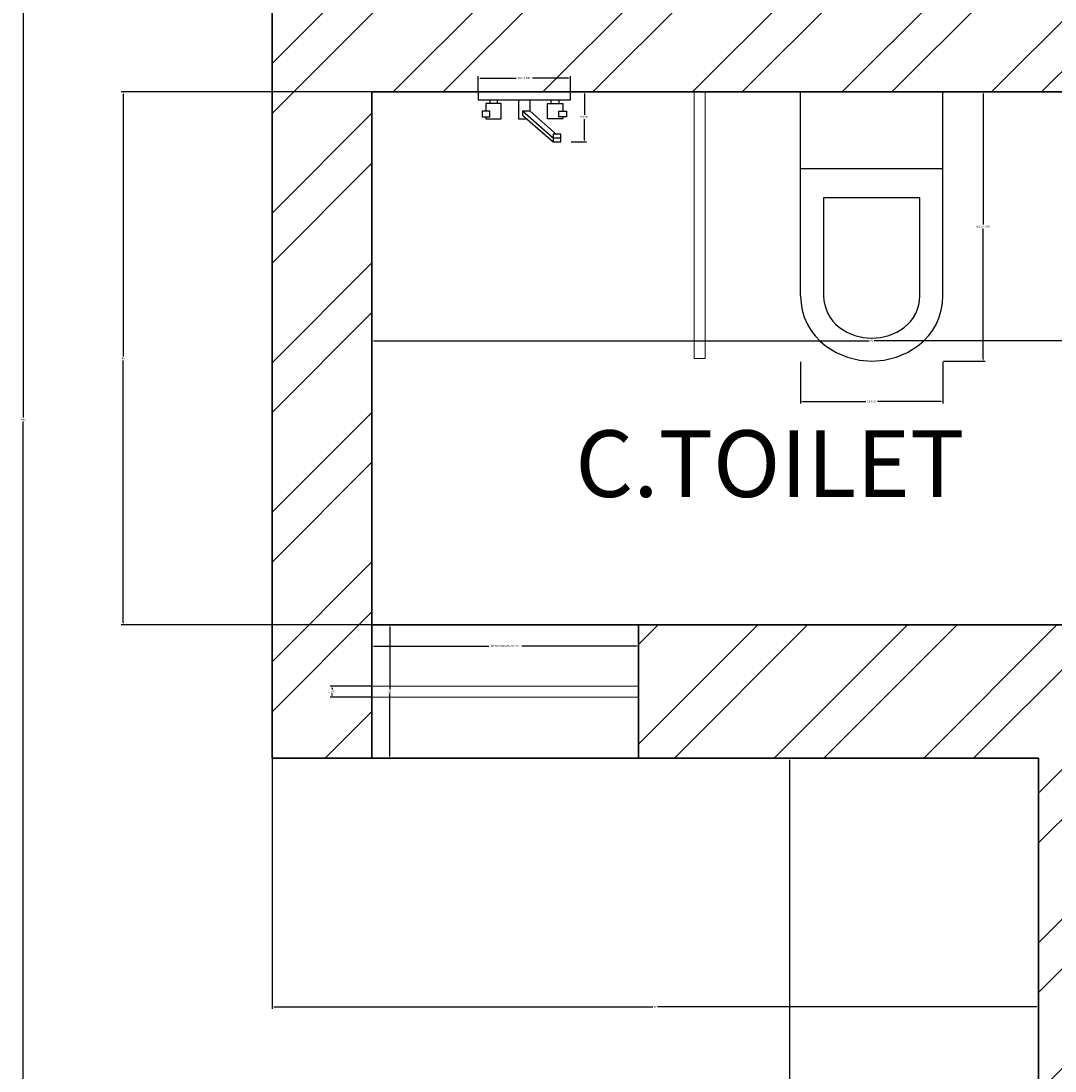
# Model space of a CAD drawing. Units: inches. Extents: x 3449 to 3843, y 1566 to 2054.
# Tile 2 of 8: x 3449 to 3543, y 1751 to 1846. Entities that reach past the tile are written whole.
import ezdxf

# ---------------------------------------------------------------- set-up
doc = ezdxf.new("R2010")
doc.units = ezdxf.units.IN
for name, color, linetype, lineweight in [('A-ANNO-DIMS', 2, 'Continuous', 18), ('A-AREA-IDEN', 7, 'Continuous', 25), ('A-GLAZ', 5, 'Continuous', 18), ('A-WALL', 7, 'Continuous', 35), ('A-WALL-PATT', 251, 'Continuous', 13), ('Сантехника', 7, 'Continuous', 18)]:
    doc.layers.add(name, color=color, linetype=linetype, lineweight=lineweight)
doc.layers.add('SANTEH', color=7, linetype='Continuous')
doc.styles.get("Standard").update_dxf_attribs({"font": 'arial.ttf'})
doc.dimstyles.get("Standard").update_dxf_attribs({"dimtxt": 0.18, "dimasz": 0.18, "dimexe": 0.18, "dimexo": 0.0625, "dimgap": 0.09, "dimtad": 0, "dimtih": 1, "dimtoh": 1, "dimdec": 4, "dimzin": 0, "dimdsep": 46, "dimtxsty": 'Standard', "dimcen": 0.09, "dimadec": 0, "dimazin": 0, "dimtfac": 1, "dimtdec": 4, "dimtofl": 0, "dimtmove": 0, "dimatfit": 3, "dimfxl": 1, "dimtolj": 1, "dimtzin": 0, "dimarcsym": 0})

# ---------------------------------------------------------------- blocks, each defined once
blk = doc.blocks.new('WC With Cistern_103')
at = {"layer": 'SANTEH'}
for p, q in [((0, 170), (0, 700)), ((370, 700), (0, 700)), ((370, 170), (370, 700)), ((370, 500), (0, 500)), ((60, 425), (60, 170)), ((310, 425), (60, 425)), ((310, 170), (310, 425))]:
    blk.add_line(p, q, dxfattribs=at)
for points in [[(0, 170), (1.1, 151.2), (4.3, 132.7), (9.7, 114.6), (17.1, 97.3), (26.5, 81), (37.7, 65.9), (50.6, 52.1), (65, 40)], [(60, 170), (60.7, 158.1), (62.7, 146.5), (66.1, 135.1), (70.8, 124.2), (76.7, 113.9), (83.8, 104.3), (91.9, 95.7), (101, 88)], [(269, 88), (278.1, 95.7), (286.2, 104.3), (293.3, 113.9), (299.2, 124.2), (303.9, 135.1), (307.3, 146.5), (309.3, 158.1), (310, 170)], [(305, 40), (319.4, 52.1), (332.3, 65.9), (343.5, 81), (352.9, 97.3), (360.3, 114.6), (365.7, 132.7), (368.9, 151.2), (370, 170)], [(101, 88), (120, 76), (140.7, 67.2), (162.6, 61.8), (185, 60), (207.4, 61.8), (229.3, 67.2), (250, 76), (269, 88)], [(65, 40), (92.2, 22.8), (121.8, 10.3), (153, 2.6), (185, 0), (217, 2.6), (248.2, 10.3), (277.8, 22.8), (305, 40)]]:
    blk.add_lwpolyline(points, dxfattribs=at)
blk = doc.blocks.new('Faucet - kit sink front')
at = {"layer": 'SANTEH'}
for p, q in [((-0.25, 3), (3.75, 6.5)), ((3.75, 6), (-0.25, 2.5)), ((4.1921, 5.5041), (0.75, 2.5)), ((3.75, 6), (3.75, 6.5)), ((3.75, 6.5), (4.75, 6.5)), ((3.75, 5.5), (3.75, 6)), ((4.75, 6), (3.75, 6)), ((4.75, 5.5), (3.75, 5.5)), ((4.75, 6.5), (4.75, 6)), ((4.75, 6), (4.75, 5.5)), ((-0.75, 3.5), (0.3192, 3.5)), ((-0.75, 1), (-0.75, 3.5)), ((-0.25, 2.5), (-0.25, 3)), ((-4.5, 1), (-4.5, 1.5)), ((-3.5, 1.5), (-3.5, 1)), ((0.75, 2.5), (-0.25, 2.5)), ((0.75, 2.5), (0.75, 1)), ((3.5, 1.5), (3.5, 1)), ((4.5, 1), (4.5, 1.5))]:
    blk.add_line(p, q, dxfattribs=at)
for points in [[(-5.5, 2.5), (-5.5, 3.25), (-4.5, 3.25), (-4.5, 2.5)], [(5.5, 2.5), (5.5, 3.25), (4.5, 3.25), (4.5, 2.5)], [(-6, 0), (-6, 1), (6, 1), (6, 0)]]:
    blk.add_lwpolyline(points, close=True, dxfattribs=at)
for points in [[(-5, 3.2513), (-5, 3.5), (-3, 3.5), (-3, 1.5), (-5, 1.5), (-5, 2.5)], [(5, 3.2513), (5, 3.5), (3, 3.5), (3, 1.5), (5, 1.5), (5, 2.5)]]:
    blk.add_lwpolyline(points, dxfattribs=at)
blk = doc.blocks.new('SHOWER-SCREEN-24')
for p, q in [((0, 24), (0, 0)), ((1, 24), (1, 0)), ((0, 0), (1, 0))]:
    blk.add_line(p, q)
blk = doc.blocks.new('GLAZING-24')
for p, q in [((24, 1), (0, 1)), ((24, 0), (0, 0))]:
    blk.add_line(p, q)
blk = doc.blocks.new('*D50')
at = {"layer": 'A-ANNO-DIMS', "color": 0, "lineweight": -2, "transparency": 16777216}
for p, q in [((3532.56, 1839.614), (3536.315, 1839.614)), ((3536.135, 1839.434), (3536.135, 1827.673)), ((3536.135, 1815.545), (3536.135, 1827.307)), ((3532.56, 1815.365), (3536.315, 1815.365))]:
    blk.add_line(p, q, dxfattribs=at)
at = {"layer": 'A-ANNO-DIMS', "color": 0, "transparency": 16777216}
for points in [[(3536.105, 1839.434), (3536.165, 1839.434), (3536.135, 1839.614)], [(3536.105, 1815.545), (3536.165, 1815.545), (3536.135, 1815.365)]]:
    blk.add_solid(points, dxfattribs=at)
at = {"layer": 'Defpoints', "color": 0, "transparency": 16777216}
for p in [(3532.497, 1839.614), (3536.135, 1839.614), (3532.497, 1815.365)]:
    blk.add_point(p, dxfattribs=at)
at = {"layer": 'A-ANNO-DIMS', "color": 0, "transparency": 16777216, "insert": (3536.135, 1827.49), "char_height": 0.18, "attachment_point": 5}
blk.add_mtext('\\A1;WC 24 TYP.', dxfattribs=at)
blk = doc.blocks.new('*D51')
at = {"layer": 'A-ANNO-DIMS', "color": 0, "lineweight": -2, "transparency": 16777216}
for p, q in [((3519.679, 1815.302), (3519.679, 1811.548)), ((3532.497, 1815.302), (3532.497, 1811.548)), ((3519.859, 1811.728), (3525.568, 1811.728)), ((3532.317, 1811.728), (3526.608, 1811.728))]:
    blk.add_line(p, q, dxfattribs=at)
at = {"layer": 'A-ANNO-DIMS', "color": 0, "transparency": 16777216}
for points in [[(3519.859, 1811.758), (3519.859, 1811.698), (3519.679, 1811.728)], [(3532.317, 1811.758), (3532.317, 1811.698), (3532.497, 1811.728)]]:
    blk.add_solid(points, dxfattribs=at)
at = {"layer": 'Defpoints', "color": 0, "transparency": 16777216}
for p in [(3519.679, 1815.365), (3532.497, 1815.365), (3532.497, 1811.728)]:
    blk.add_point(p, dxfattribs=at)
at = {"layer": 'A-ANNO-DIMS', "color": 0, "transparency": 16777216, "insert": (3526.088, 1811.728), "char_height": 0.18, "attachment_point": 5}
blk.add_mtext('\\A1;13 TYP.', dxfattribs=at)
blk = doc.blocks.new('*D52')
at = {"layer": 'A-ANNO-DIMS', "color": 0, "lineweight": -2, "transparency": 16777216}
for p, q in [((3490.648, 1839.677), (3490.648, 1841.041)), ((3490.828, 1840.861), (3494.065, 1840.861)), ((3498.782, 1840.861), (3495.544, 1840.861)), ((3498.962, 1839.677), (3498.962, 1841.041))]:
    blk.add_line(p, q, dxfattribs=at)
at = {"layer": 'A-ANNO-DIMS', "color": 0, "transparency": 16777216}
for points in [[(3490.828, 1840.891), (3490.828, 1840.831), (3490.648, 1840.861)], [(3498.782, 1840.891), (3498.782, 1840.831), (3498.962, 1840.861)]]:
    blk.add_solid(points, dxfattribs=at)
at = {"layer": 'Defpoints', "color": 0, "transparency": 16777216}
for p in [(3498.962, 1840.861), (3490.648, 1839.614), (3498.962, 1839.614)]:
    blk.add_point(p, dxfattribs=at)
at = {"layer": 'A-ANNO-DIMS', "color": 0, "transparency": 16777216, "insert": (3494.805, 1840.861), "char_height": 0.18, "attachment_point": 5}
blk.add_mtext('\\A1;TAP 8 TYP.', dxfattribs=at)
blk = doc.blocks.new('*D53')
at = {"layer": 'A-ANNO-DIMS', "color": 0, "lineweight": -2, "transparency": 16777216}
for p, q in [((3499.024, 1839.614), (3500.389, 1839.614)), ((3500.209, 1839.434), (3500.209, 1837.544)), ((3500.209, 1835.291), (3500.209, 1837.181)), ((3499.024, 1835.111), (3500.389, 1835.111))]:
    blk.add_line(p, q, dxfattribs=at)
at = {"layer": 'A-ANNO-DIMS', "color": 0, "transparency": 16777216}
for points in [[(3500.179, 1839.434), (3500.239, 1839.434), (3500.209, 1839.614)], [(3500.179, 1835.291), (3500.239, 1835.291), (3500.209, 1835.111)]]:
    blk.add_solid(points, dxfattribs=at)
at = {"layer": 'Defpoints', "color": 0, "transparency": 16777216}
for p in [(3498.962, 1839.614), (3498.962, 1835.111), (3500.209, 1835.111)]:
    blk.add_point(p, dxfattribs=at)
at = {"layer": 'A-ANNO-DIMS', "color": 0, "transparency": 16777216, "insert": (3500.209, 1837.363), "char_height": 0.18, "attachment_point": 5}
blk.add_mtext('\\A1;5 TYP.', dxfattribs=at)
blk = doc.blocks.new('*D58')
at = {"layer": 'A-ANNO-DIMS', "color": 0, "lineweight": -2, "transparency": 16777216}
for p, q in [((3481.088, 1786.177), (3481.088, 1789.894)), ((3481.268, 1789.714), (3491.607, 1789.714)), ((3504.908, 1789.714), (3494.569, 1789.714)), ((3505.088, 1786.177), (3505.088, 1789.894))]:
    blk.add_line(p, q, dxfattribs=at)
at = {"layer": 'A-ANNO-DIMS', "color": 0, "transparency": 16777216}
for points in [[(3481.268, 1789.744), (3481.268, 1789.684), (3481.088, 1789.714)], [(3504.908, 1789.744), (3504.908, 1789.684), (3505.088, 1789.714)]]:
    blk.add_solid(points, dxfattribs=at)
at = {"layer": 'Defpoints', "color": 0, "transparency": 16777216}
for p in [(3505.088, 1789.714), (3481.088, 1786.114), (3505.088, 1786.114)]:
    blk.add_point(p, dxfattribs=at)
at = {"layer": 'A-ANNO-DIMS', "color": 0, "transparency": 16777216, "insert": (3493.088, 1789.714), "char_height": 0.18, "attachment_point": 5}
blk.add_mtext('\\A1;BATH WINDOW 24 TYP.', dxfattribs=at)
blk = doc.blocks.new('*D59')
at = {"layer": 'A-ANNO-DIMS', "color": 0, "lineweight": -2, "transparency": 16777216}
for p, q in [((3481.026, 1786.114), (3477.308, 1786.114)), ((3477.488, 1785.934), (3477.488, 1785.795)), ((3477.488, 1785.294), (3477.488, 1785.434)), ((3481.026, 1785.114), (3477.308, 1785.114))]:
    blk.add_line(p, q, dxfattribs=at)
at = {"layer": 'A-ANNO-DIMS', "color": 0, "transparency": 16777216}
for points in [[(3477.458, 1785.934), (3477.518, 1785.934), (3477.488, 1786.114)], [(3477.458, 1785.294), (3477.518, 1785.294), (3477.488, 1785.114)]]:
    blk.add_solid(points, dxfattribs=at)
at = {"layer": 'Defpoints', "color": 0, "transparency": 16777216}
for p in [(3477.488, 1786.114), (3481.088, 1786.114), (3481.088, 1785.114)]:
    blk.add_point(p, dxfattribs=at)
at = {"layer": 'A-ANNO-DIMS', "color": 0, "transparency": 16777216, "insert": (3477.488, 1785.614), "char_height": 0.18, "attachment_point": 5}
blk.add_mtext('\\A1;1 TYP.', dxfattribs=at)
blk = doc.blocks.new('*D77')
at = {"layer": 'A-ANNO-DIMS', "color": 0, "lineweight": -2, "transparency": 16777216}
for p, q in [((3472.026, 2031.614), (3449.508, 2031.614)), ((3449.688, 2031.434), (3449.688, 1810.296)), ((3449.688, 1588.794), (3449.688, 1809.932)), ((3481.026, 1588.614), (3449.508, 1588.614))]:
    blk.add_line(p, q, dxfattribs=at)
at = {"layer": 'A-ANNO-DIMS', "color": 0, "transparency": 16777216}
for points in [[(3449.658, 2031.434), (3449.718, 2031.434), (3449.688, 2031.614)], [(3449.658, 1588.794), (3449.718, 1588.794), (3449.688, 1588.614)]]:
    blk.add_solid(points, dxfattribs=at)
at = {"layer": 'Defpoints', "color": 0, "transparency": 16777216}
for p in [(3449.688, 2031.614), (3472.088, 2031.614), (3481.088, 1588.614)]:
    blk.add_point(p, dxfattribs=at)
at = {"layer": 'A-ANNO-DIMS', "color": 0, "transparency": 16777216, "insert": (3449.688, 1810.114), "char_height": 0.18, "attachment_point": 5}
blk.add_mtext('\\A1;443', dxfattribs=at)
blk = doc.blocks.new('*D89')
at = {"layer": 'A-ANNO-DIMS', "color": 0, "lineweight": -2, "transparency": 16777216}
for p, q in [((3481.088, 1839.552), (3481.088, 1817.034)), ((3571.088, 1839.552), (3571.088, 1817.034)), ((3481.268, 1817.214), (3525.869, 1817.214)), ((3570.908, 1817.214), (3526.307, 1817.214))]:
    blk.add_line(p, q, dxfattribs=at)
at = {"layer": 'A-ANNO-DIMS', "color": 0, "transparency": 16777216}
for points in [[(3481.268, 1817.244), (3481.268, 1817.184), (3481.088, 1817.214)], [(3570.908, 1817.244), (3570.908, 1817.184), (3571.088, 1817.214)]]:
    blk.add_solid(points, dxfattribs=at)
at = {"layer": 'Defpoints', "color": 0, "transparency": 16777216}
for p in [(3481.088, 1839.614), (3571.088, 1839.614), (3481.088, 1817.214)]:
    blk.add_point(p, dxfattribs=at)
at = {"layer": 'A-ANNO-DIMS', "color": 0, "transparency": 16777216, "insert": (3526.088, 1817.214), "char_height": 0.18, "attachment_point": 5}
blk.add_mtext('\\A1;90', dxfattribs=at)
blk = doc.blocks.new('*D90')
at = {"layer": 'A-ANNO-DIMS', "color": 0, "lineweight": -2, "transparency": 16777216}
for p, q in [((3481.026, 1839.614), (3458.508, 1839.614)), ((3458.688, 1839.434), (3458.688, 1815.796)), ((3458.688, 1791.794), (3458.688, 1815.432)), ((3481.026, 1791.614), (3458.508, 1791.614))]:
    blk.add_line(p, q, dxfattribs=at)
at = {"layer": 'A-ANNO-DIMS', "color": 0, "transparency": 16777216}
for points in [[(3458.658, 1839.434), (3458.718, 1839.434), (3458.688, 1839.614)], [(3458.658, 1791.794), (3458.718, 1791.794), (3458.688, 1791.614)]]:
    blk.add_solid(points, dxfattribs=at)
at = {"layer": 'Defpoints', "color": 0, "transparency": 16777216}
for p in [(3458.688, 1839.614), (3481.088, 1839.614), (3481.088, 1791.614)]:
    blk.add_point(p, dxfattribs=at)
at = {"layer": 'A-ANNO-DIMS', "color": 0, "transparency": 16777216, "insert": (3458.688, 1815.614), "char_height": 0.18, "attachment_point": 5}
blk.add_mtext('\\A1;48', dxfattribs=at)
blk = doc.blocks.new('*D95')
at = {"layer": 'A-ANNO-DIMS', "color": 0, "lineweight": -2, "transparency": 16777216}
for p, q in [((3472.088, 1779.552), (3472.088, 1757.034)), ((3541.088, 1779.552), (3541.088, 1757.034)), ((3472.268, 1757.214), (3506.368, 1757.214)), ((3540.908, 1757.214), (3506.808, 1757.214))]:
    blk.add_line(p, q, dxfattribs=at)
at = {"layer": 'A-ANNO-DIMS', "color": 0, "transparency": 16777216}
for points in [[(3472.268, 1757.244), (3472.268, 1757.184), (3472.088, 1757.214)], [(3540.908, 1757.244), (3540.908, 1757.184), (3541.088, 1757.214)]]:
    blk.add_solid(points, dxfattribs=at)
at = {"layer": 'Defpoints', "color": 0, "transparency": 16777216}
for p in [(3472.088, 1779.614), (3541.088, 1779.614), (3472.088, 1757.214)]:
    blk.add_point(p, dxfattribs=at)
at = {"layer": 'A-ANNO-DIMS', "color": 0, "transparency": 16777216, "insert": (3506.588, 1757.214), "char_height": 0.18, "attachment_point": 5}
blk.add_mtext('\\A1;69', dxfattribs=at)
blk = doc.blocks.new('*D96')
at = {"layer": 'A-ANNO-DIMS', "color": 0, "lineweight": -2, "transparency": 16777216}
for p, q in [((3541.026, 1779.614), (3518.508, 1779.614)), ((3518.688, 1779.434), (3518.688, 1718.795)), ((3518.688, 1657.794), (3518.688, 1718.434)), ((3541.026, 1657.614), (3518.508, 1657.614))]:
    blk.add_line(p, q, dxfattribs=at)
at = {"layer": 'A-ANNO-DIMS', "color": 0, "transparency": 16777216}
for points in [[(3518.658, 1779.434), (3518.718, 1779.434), (3518.688, 1779.614)], [(3518.658, 1657.794), (3518.718, 1657.794), (3518.688, 1657.614)]]:
    blk.add_solid(points, dxfattribs=at)
at = {"layer": 'Defpoints', "color": 0, "transparency": 16777216}
for p in [(3518.688, 1779.614), (3541.088, 1779.614), (3541.088, 1657.614)]:
    blk.add_point(p, dxfattribs=at)
at = {"layer": 'A-ANNO-DIMS', "color": 0, "transparency": 16777216, "insert": (3518.688, 1718.614), "char_height": 0.18, "attachment_point": 5}
blk.add_mtext('\\A1;122', dxfattribs=at)
blk = doc.blocks.new('*D113')
at = {"layer": 'A-ANNO-DIMS', "color": 0, "lineweight": -2, "transparency": 16777216}
for p, q in [((3505.026, 1791.614), (3482.508, 1791.614)), ((3482.688, 1791.434), (3482.688, 1785.795)), ((3482.688, 1779.794), (3482.688, 1785.434)), ((3505.026, 1779.614), (3482.508, 1779.614))]:
    blk.add_line(p, q, dxfattribs=at)
at = {"layer": 'A-ANNO-DIMS', "color": 0, "transparency": 16777216}
for points in [[(3482.658, 1791.434), (3482.718, 1791.434), (3482.688, 1791.614)], [(3482.658, 1779.794), (3482.718, 1779.794), (3482.688, 1779.614)]]:
    blk.add_solid(points, dxfattribs=at)
at = {"layer": 'Defpoints', "color": 0, "transparency": 16777216}
for p in [(3482.688, 1791.614), (3505.088, 1791.614), (3505.088, 1779.614)]:
    blk.add_point(p, dxfattribs=at)
at = {"layer": 'A-ANNO-DIMS', "color": 0, "transparency": 16777216, "insert": (3482.688, 1785.614), "char_height": 0.18, "attachment_point": 5}
blk.add_mtext('\\A1;12', dxfattribs=at)

msp = doc.modelspace()

# ---------------------------------------------------------------- hatches: boundary and pattern name
at = {"layer": 'A-WALL-PATT'}
h = msp.add_hatch(dxfattribs=at)
h.set_pattern_fill('ANSI32', color=256)
edge = h.paths.add_edge_path()
edge.add_line((3481.088, 2022.6144), (3508.088, 2022.6144))
edge.add_line((3508.088, 2022.6144), (3508.088, 2031.6144))
edge.add_line((3508.088, 2031.6144), (3472.088, 2031.6144))
edge.add_line((3472.088, 2031.6144), (3472.088, 1779.6144))
edge.add_line((3472.088, 1779.6144), (3481.088, 1779.6144))
edge.add_line((3481.088, 1779.6144), (3481.088, 1839.6144))
edge.add_line((3481.088, 1839.6144), (3571.088, 1839.6144))
edge.add_line((3571.088, 1839.6144), (3571.088, 1824.3194))
edge.add_line((3571.088, 1824.3194), (3571.088, 1821.6144))
edge.add_line((3571.088, 1821.6144), (3580.088, 1821.6144))
edge.add_line((3580.088, 1821.6144), (3580.088, 1825.1908))
edge.add_ellipse((3580.1411, 1825.2442), major_axis=(0, 0.0754), ratio=0.9991395, start_angle=90, end_angle=135.183195, ccw=False)
edge.add_line((3580.0017, 1825.3196), (3580.0658, 1825.3196))
edge.add_line((3580.0658, 1825.3196), (3580.066, 1839.6365))
edge.add_line((3580.066, 1839.6365), (3616.088, 1839.6365))
edge.add_line((3616.088, 1839.6365), (3616.088, 1848.6144))
edge.add_line((3616.088, 1848.6144), (3610.088, 1848.6144))
edge.add_line((3610.088, 1848.6144), (3574.088, 1848.6144))
edge.add_line((3574.088, 1848.6144), (3481.088, 1848.6144))
edge.add_line((3481.088, 1848.6144), (3481.088, 1872.6144))
edge.add_line((3481.088, 1872.6144), (3481.088, 2022.6144))
h.paths.add_polyline_path([(3550.088, 1779.6144), (3616.088, 1779.6144), (3616.088, 1791.6144), (3505.088, 1791.6144), (3505.088, 1779.6144), (3541.088, 1779.6144), (3541.088, 1657.6144), (3481.088, 1657.6144), (3481.088, 1588.6144), (3496.088, 1588.6144), (3496.088, 1594.6144), (3496.088, 1597.6144), (3490.088, 1597.6144), (3490.088, 1648.6144), (3550.088, 1648.6144)])
h.paths.add_polyline_path([(3775.088, 1612.6144), (3766.088, 1612.6144), (3766.088, 1597.6144), (3536.088, 1597.6144), (3536.088, 1588.6144), (3775.088, 1588.6144)])
h.paths.add_polyline_path([(3820.088, 1756.6144), (3811.088, 1756.6144), (3811.088, 1732.6144), (3664.088, 1732.6144), (3664.088, 1723.6144), (3766.088, 1723.6144), (3766.088, 1708.6144), (3775.088, 1708.6144), (3775.088, 1723.6144), (3820.088, 1723.6144)])
h.paths.add_polyline_path([(3820.088, 1986.6144), (3745.088, 1986.6144), (3745.088, 2010.6144), (3664.088, 2010.6144), (3664.088, 1992.6144), (3652.088, 1992.6144), (3652.088, 1983.6144), (3664.088, 1983.6144), (3664.088, 1893.6144), (3648.793, 1893.6144), (3607.088, 1893.6144), (3607.088, 1884.6144), (3673.088, 1884.6144), (3673.088, 2001.6144), (3736.088, 2001.6144), (3736.088, 1977.6144), (3811.088, 1977.6144), (3811.088, 1949.1144), (3820.088, 1949.1144)])
h.paths.add_polyline_path([(3628.088, 1992.6144), (3616.088, 1992.6144), (3616.088, 2031.6144), (3580.088, 2031.6144), (3580.088, 2022.6144), (3607.088, 2022.6144), (3607.088, 1921.6144), (3613.088, 1921.6144), (3616.088, 1921.6144), (3616.088, 1983.6144), (3628.088, 1983.6144)])
h.paths.add_polyline_path([(3820.088, 1877.1144), (3811.088, 1877.1144), (3811.088, 1848.6144), (3664.088, 1848.6144), (3664.088, 1839.6144), (3700.088, 1839.6144), (3811.088, 1839.6144), (3811.088, 1815.6144), (3820.088, 1815.6144)])

# ---------------------------------------------------------------- linework, layer by layer
at = {"layer": 'A-WALL'}
for p, q in [((3472.088, 2031.6144), (3472.088, 1779.6144)), ((3481.088, 1839.6144), (3571.088, 1839.6144)), ((3481.088, 1839.6144), (3481.088, 1779.6144)), ((3481.088, 1791.6144), (3616.088, 1791.6144)), ((3505.088, 1791.6144), (3505.088, 1779.6144)), ((3472.088, 1779.6144), (3481.088, 1779.6144)), ((3481.088, 1779.6144), (3541.088, 1779.6144)), ((3541.088, 1779.6144), (3541.088, 1657.6144))]:
    msp.add_line(p, q, dxfattribs=at)

# ---------------------------------------------------------------- block references
at = {"layer": 'A-GLAZ'}
msp.add_blockref('GLAZING-24', (3481.088, 1785.114), dxfattribs=at)
at = {"layer": 'Сантехника', "xscale": -0.6928340246039085, "yscale": 0.6928340246039085, "zscale": 0.6928340246039085, "rotation": 180}
msp.add_blockref('Faucet - kit sink front', (3494.8045, 1839.6144), dxfattribs=at)
at = {"layer": 'Сантехника'}
msp.add_blockref('SHOWER-SCREEN-24', (3510.088, 1815.614), dxfattribs=at)
at = {"layer": 'Сантехника', "xscale": 0.0346417012301954, "yscale": 0.0346417012301954, "zscale": 0.0346417012301954}
msp.add_blockref('WC With Cistern_103', (3519.6793, 1815.3652), dxfattribs=at)

# ---------------------------------------------------------------- texts
at = {"layer": 'A-AREA-IDEN', "insert": (3499.3923, 1809.1393), "char_height": 6, "attachment_point": 1}
msp.add_mtext_dynamic_manual_height_columns('C.TOILET', width=95.638287, gutter_width=12.5, heights=[0], dxfattribs=at)

# ---------------------------------------------------------------- dimensions: what is measured, and where the dimension line sits
at = {"layer": 'A-ANNO-DIMS'}
for base, p1, p2, angle, picture, middle in [((3449.688, 2031.6144), (3481.088, 1588.6144), (3472.088, 2031.6144), 90, '*D77', (3449.688, 1810.1144)), ((3458.688, 1839.6144), (3481.088, 1791.6144), (3481.088, 1839.6144), 90, '*D90', (3458.688, 1815.6144)), ((3481.088, 1817.2144), (3571.088, 1839.6144), (3481.088, 1839.6144), 180, '*D89', (3526.088, 1817.2144)), ((3482.688, 1791.6144), (3505.088, 1779.6144), (3505.088, 1791.6144), 90, '*D113', (3482.688, 1785.6144)), ((3472.088, 1757.2144), (3541.088, 1779.6144), (3472.088, 1779.6144), 180, '*D95', (3506.588, 1757.2144)), ((3518.688, 1779.6144), (3541.088, 1657.6144), (3541.088, 1779.6144), 90, '*D96', (3518.688, 1718.6144))]:
    dim = msp.add_linear_dim(base=base, p1=p1, p2=p2, angle=angle, dimstyle='Standard', override={"dimdec": 0, "dimlfac": 1, "dimrnd": 0, "dimzin": 0, "dimdsep": 46, "dimlunit": 2}, dxfattribs=at)
    dim.commit()
    dim.dimension.update_dxf_attribs({"geometry": picture, "text_midpoint": middle})
for base, p1, p2, text, picture, middle in [((3498.9615, 1840.8615), (3490.6475, 1839.6144), (3498.9615, 1839.6144), 'TAP <> TYP.', '*D52', (3494.8045, 1840.8615)), ((3532.4973, 1811.7276), (3519.6787, 1815.365), (3532.4973, 1815.365), '<> TYP.', '*D51', (3526.088, 1811.7276)), ((3505.088, 1789.7144), (3481.088, 1786.1144), (3505.088, 1786.1144), 'BATH WINDOW <> TYP.', '*D58', (3493.088, 1789.7144))]:
    dim = msp.add_linear_dim(base=base, p1=p1, p2=p2, text=text, dimstyle='Standard', override={"dimdec": 0, "dimlfac": 1, "dimrnd": 0, "dimzin": 0, "dimdsep": 46, "dimlunit": 2}, dxfattribs=at)
    dim.commit()
    dim.dimension.update_dxf_attribs({"geometry": picture, "text_midpoint": middle})
for base, p1, p2, angle, text, picture, middle in [((3500.2086, 1835.111), (3498.9615, 1839.6144), (3498.9615, 1835.111), 270, '<> TYP.', '*D53', (3500.2086, 1837.3627)), ((3536.1347, 1839.6144), (3532.4973, 1815.365), (3532.4973, 1839.6144), 90, 'WC <> TYP.', '*D50', (3536.1347, 1827.4897)), ((3477.488, 1786.1144), (3481.088, 1785.1144), (3481.088, 1786.1144), 90, '<> TYP.', '*D59', (3477.488, 1785.6144))]:
    dim = msp.add_linear_dim(base=base, p1=p1, p2=p2, angle=angle, text=text, dimstyle='Standard', override={"dimdec": 0, "dimlfac": 1, "dimrnd": 0, "dimzin": 0, "dimdsep": 46, "dimlunit": 2}, dxfattribs=at)
    dim.commit()
    dim.dimension.update_dxf_attribs({"geometry": picture, "text_midpoint": middle})

doc.saveas('drawing.dxf')
